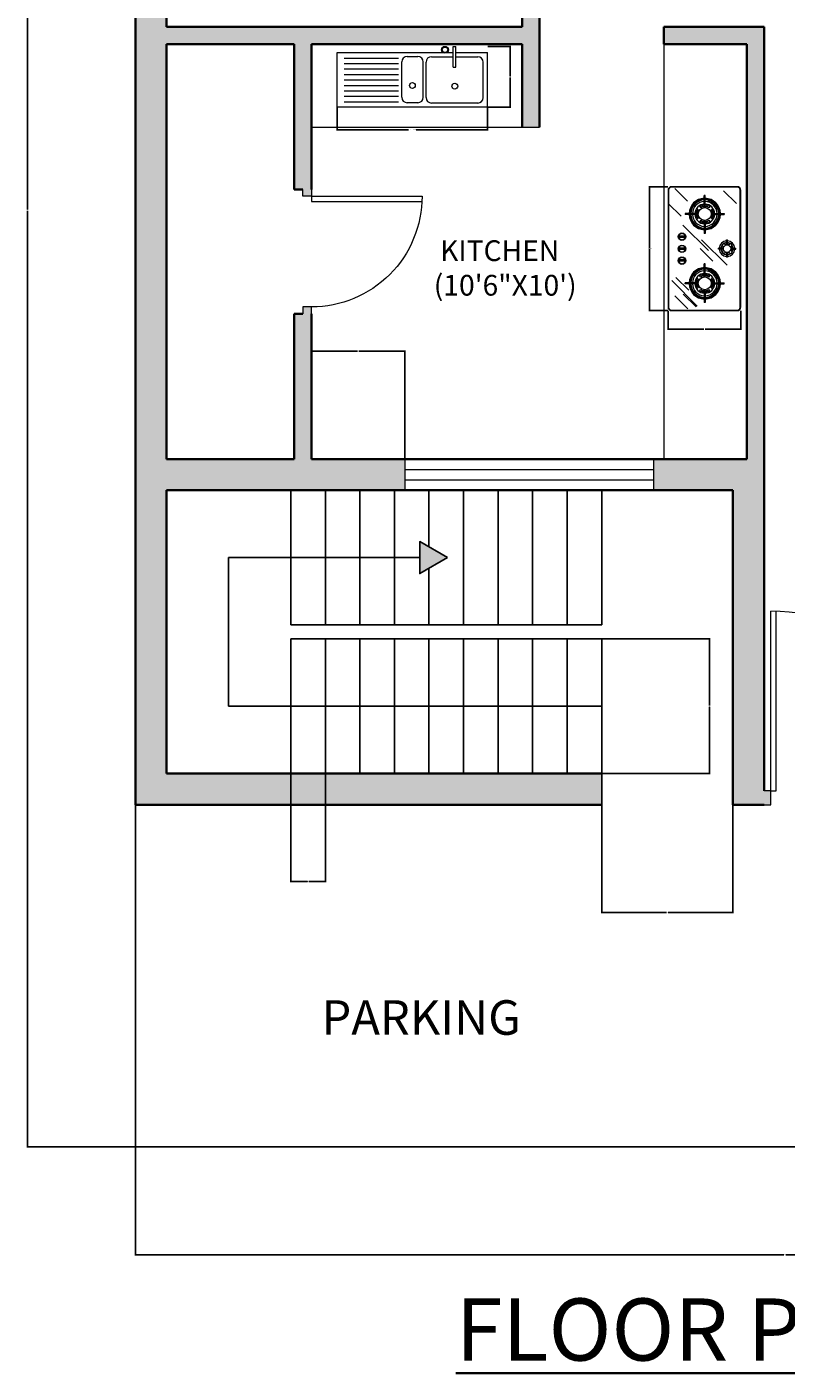
# Model space of a CAD drawing. Units: inches. Extents: x 2948 to 4025, y 2171 to 2966.
# Tile 1 of 6: x 2948 to 3168, y 2171 to 2560. Entities that reach past the tile are written whole.
import ezdxf

# ---------------------------------------------------------------- set-up
doc = ezdxf.new("R2010")
doc.units = ezdxf.units.IN
for name, color, linetype, lineweight in [('A-ANNO-DIMS', 2, 'Continuous', 18), ('A-ANNO-TEXT', 7, 'Continuous', 35), ('A-AREA-IDEN', 7, 'Continuous', 18), ('A-DOOR', 3, 'Continuous', 18), ('A-EQPM', 8, 'Continuous', 18), ('A-FLOR-CASE', 8, 'Continuous', 18), ('A-FLOR-FIXT', 9, 'Continuous', 18), ('A-FLOR-STRS', 7, 'Continuous', 25), ('A-GLAZ', 4, 'Continuous', 18), ('A-WALL', 7, 'Continuous', 35), ('A-WALL-PATT', 252, 'Continuous', 13)]:
    doc.layers.add(name, color=color, linetype=linetype, lineweight=lineweight)
doc.styles.get("Standard").update_dxf_attribs({"font": 'arial.ttf'})
doc.dimstyles.get("Standard").update_dxf_attribs({"dimtxt": 0.18, "dimasz": 0.18, "dimexe": 0.18, "dimexo": 0.0625, "dimgap": 0.09, "dimtad": 0, "dimtih": 1, "dimtoh": 1, "dimdec": 4, "dimzin": 0, "dimdsep": 46, "dimtxsty": 'Standard', "dimcen": 0.09, "dimadec": 0, "dimazin": 0, "dimtfac": 1, "dimtdec": 4, "dimtofl": 0, "dimtmove": 0, "dimatfit": 3, "dimfxl": 1, "dimtolj": 1, "dimtzin": 0, "dimarcsym": 0})

# ---------------------------------------------------------------- blocks, each defined once
blk = doc.blocks.new('A$C038F079D')
for p, q in [((23.9, 336.8), (101.3, 414.2)), ((377.5, 410.6), (372.5, 410.6)), ((320.9, 202.7), (475.7, 357.5)), ((427.1, 359.8), (427.1, 354.8)), ((587.4, 339.9), (582.4, 339.9)), ((377.5, 305.6), (372.5, 305.6)), ((374.2, 193.8), (451.6, 271.2)), ((53.2, 224.7), (53.2, 219.7)), ((130.3, 173.3), (141.1, 184.1)), ((137.3, 169), (142.6, 174.2)), ((232.1, 89.3), (386.9, 244.1)), ((284, 224.7), (284, 219.7)), ((466, 224.7), (466, 219.7)), ((567.6, 22.2), (722.4, 177)), ((650.5, 92.2), (727.9, 169.6)), ((701.8, 224.7), (701.8, 219.7)), ((10.1, 41), (87.5, 118.4)), ((549.9, 47.9), (627.2, 125.3)), ((587.4, 103.7), (582.4, 103.7)), ((661.4, 42), (738.7, 119.3)), ((100.9, 1.5), (178.3, 78.9))]:
    blk.add_line(p, q)
at = {"ltscale": 0.18}
for p, q in [((372.5, 384.7), (372.5, 410.6)), ((377.5, 384.7), (377.5, 410.6)), ((162.6, 339.9), (167.6, 339.9)), ((162.6, 267.1), (162.6, 339.9)), ((167.6, 267.1), (167.6, 339.9)), ((322.3, 354.8), (322.3, 359.8)), ((347.6, 359.8), (322.3, 359.8)), ((347.6, 354.8), (322.3, 354.8)), ((350.8, 370.2), (343.5, 377.5)), ((343.5, 337.2), (350.8, 344.5)), ((362.2, 381.5), (354.8, 388.8)), ((354.8, 325.8), (362.2, 333.1)), ((372.5, 329.9), (372.5, 305.6)), ((377.5, 329.9), (377.5, 305.6)), ((387.8, 381.5), (395.2, 388.8)), ((395.2, 325.8), (387.8, 333.1)), ((399.2, 370.2), (406.5, 377.5)), ((406.5, 337.2), (399.2, 344.5)), ((402.4, 359.8), (427.1, 359.8)), ((402.4, 354.8), (427.1, 354.8)), ((582.4, 267.1), (582.4, 339.9)), ((587.4, 267.1), (587.4, 339.9)), ((111.9, 250), (117.1, 244.7)), ((116.2, 257), (127, 246.2)), ((130.3, 271.1), (141.1, 260.3)), ((137.3, 275.4), (142.6, 270.2)), ((187.6, 270.2), (192.8, 275.4)), ((189, 260.3), (199.8, 271.1)), ((203.2, 246.2), (214, 257)), ((213.1, 244.7), (218.3, 250)), ((536.9, 244.7), (531.7, 250)), ((546.8, 246.2), (536, 257)), ((561, 260.3), (550.2, 271.1)), ((562.4, 270.2), (557.2, 275.4)), ((612.7, 275.4), (607.4, 270.2)), ((619.7, 271.1), (608.9, 260.3)), ((633.8, 257), (623, 246.2)), ((638.1, 250), (632.9, 244.7)), ((125.1, 224.7), (53.2, 224.7)), ((125.1, 219.7), (53.2, 219.7)), ((111.9, 194.5), (117.1, 199.7)), ((116.2, 187.5), (127, 198.3)), ((162.6, 177.3), (162.6, 103.7)), ((167.6, 177.3), (167.6, 103.7)), ((187.6, 174.2), (192.8, 169)), ((189, 184.1), (199.8, 173.3)), ((203.2, 198.3), (214, 187.5)), ((210, 224.7), (284, 224.7)), ((210, 219.7), (284, 219.7)), ((213.1, 199.7), (218.3, 194.5)), ((540, 224.7), (466, 224.7)), ((540, 219.7), (466, 219.7)), ((536.9, 199.7), (531.7, 194.5)), ((546.8, 198.3), (536, 187.5)), ((561, 184.1), (550.2, 173.3)), ((562.4, 174.2), (557.2, 169)), ((582.4, 177.3), (582.4, 103.7)), ((587.4, 177.3), (587.4, 103.7)), ((612.7, 169), (607.4, 174.2)), ((619.7, 173.3), (608.9, 184.1)), ((633.8, 187.5), (623, 198.3)), ((629.9, 224.7), (701.8, 224.7)), ((629.9, 219.7), (701.8, 219.7)), ((638.1, 194.5), (632.9, 199.7)), ((162.6, 103.7), (167.6, 103.7)), ((298.6, 99.8), (298.6, 69)), ((306.6, 99.8), (306.6, 69)), ((372, 99.8), (372, 69)), ((380, 99.8), (380, 69)), ((443.4, 99.8), (443.4, 69)), ((451.4, 99.8), (451.4, 69))]:
    blk.add_line(p, q, dxfattribs=at)
for points in [[(20, 0), (730, 0, 0.414214), (750, 20), (750, 420, 0.414214), (730, 440), (20, 440, 0.414214), (0, 420), (0, 20, 0.414214)], [(20, 3), (730, 3, 0.414214), (747, 20), (747, 420, 0.414214), (730, 437), (20, 437, 0.414214), (3, 420), (3, 20, 0.414214)]]:
    blk.add_lwpolyline(points, format="xyb", close=True)
for centre in [(345.9, 386.3), (89.1, 248.3), (94.7, 261.5), (509, 247.6), (514.6, 260.8)]:
    blk.add_circle(centre, 3.73)
for centre, radius in [((375, 357.3), 22.4), ((165.1, 222.2), 39), ((584.9, 222.2), 39), ((302.6, 84.4), 22.5), ((302.6, 84.4), 21.5), ((376, 84.4), 22.5), ((376, 84.4), 21.5), ((447.4, 84.4), 22.5), ((447.4, 84.4), 21.5)]:
    blk.add_circle(centre, radius, dxfattribs=at)
for centre, radius, start, end in [((375, 357.3), 47.4, 93.02552, 176.97448), ((375, 357.3), 47.4, 183.02552, 266.97448), ((375, 357.3), 37.4, 93.83631, 176.16369), ((375, 357.3), 37.4, 183.83631, 266.16369), ((346.8, 357.3), 2.62, 287.63178, 72.36822), ((375, 357.3), 27.4, 151.9979, 174.83836), ((375, 357.3), 27.4, 185.16164, 208.0021), ((375, 357.3), 27.4, 95.20298, 118.0021), ((375, 357.3), 27.4, 241.9979, 264.75693), ((375, 385), 2.52, 187.95053, 352.04947), ((375, 330), 2.5, 358.33173, 181.66827), ((375, 357.3), 47.4, 3.02552, 86.97448), ((375, 357.3), 37.4, 3.83631, 86.16369), ((375, 357.3), 27.4, 61.9979, 84.79702), ((375, 357.3), 47.4, 273.02552, 356.97448), ((375, 357.3), 37.4, 273.83631, 356.16369), ((375, 357.3), 27.4, 275.24307, 298.0021), ((375, 357.3), 27.4, 5.20601, 28.0021), ((375, 357.3), 27.4, 331.9979, 354.79399), ((402.7, 357.3), 2.52, 97.22361, 262.77639), ((165.1, 222.2), 95, 91.59175, 178.40825), ((165.1, 222.2), 90, 91.59175, 178.40825), ((165.1, 222.2), 85, 91.68541, 178.31459), ((165.1, 222.2), 75, 91.91021, 178.08979), ((165.1, 222.2), 60, 92.38802, 177.61198), ((165.1, 222.2), 53, 154.85389, 177.29637), ((165.1, 222.2), 45, 147.83959, 176.81526), ((165.1, 222.2), 45, 93.18474, 122.16041), ((165.1, 222.2), 53, 92.70363, 115.14611), ((165.1, 267.4), 2.52, 186.73537, 353.26463), ((165.1, 222.2), 90, 1.59175, 88.40825), ((165.1, 222.2), 85, 1.68541, 88.31459), ((165.1, 222.2), 75, 1.91021, 88.08979), ((165.1, 222.2), 60, 2.38802, 87.61198), ((165.1, 222.2), 53, 64.85389, 87.29637), ((165.1, 222.2), 45, 57.83959, 86.81526), ((165.1, 222.2), 95, 1.59175, 88.40825), ((165.1, 222.2), 45, 3.18474, 32.16041), ((165.1, 222.2), 53, 2.70363, 25.14611), ((584.9, 222.2), 95, 91.59175, 178.40825), ((584.9, 222.2), 90, 91.59175, 178.40825), ((584.9, 222.2), 85, 91.68541, 178.31459), ((584.9, 222.2), 75, 91.91021, 178.08979), ((584.9, 222.2), 60, 92.38802, 177.61198), ((584.9, 222.2), 53, 154.85389, 177.29637), ((584.9, 222.2), 45, 147.83959, 176.81526), ((584.9, 222.2), 45, 93.18474, 122.16041), ((584.9, 222.2), 53, 92.70363, 115.14611), ((584.9, 267.3), 2.51, 183.95793, 356.04207), ((584.9, 222.2), 90, 1.59175, 88.40825), ((584.9, 222.2), 85, 1.68541, 88.31459), ((584.9, 222.2), 75, 1.91021, 88.08979), ((584.9, 222.2), 60, 2.38802, 87.61198), ((584.9, 222.2), 53, 64.85389, 87.29637), ((584.9, 222.2), 45, 57.83959, 86.81526), ((584.9, 222.2), 95, 1.59175, 88.40825), ((584.9, 222.2), 45, 3.18474, 32.16041), ((584.9, 222.2), 53, 2.70363, 25.14611), ((165.1, 222.2), 95, 181.59175, 268.40825), ((165.1, 222.2), 90, 181.59175, 268.40825), ((165.1, 222.2), 85, 181.68541, 268.31459), ((165.1, 222.2), 75, 181.91021, 268.08979), ((165.1, 222.2), 60, 182.38802, 267.61198), ((165.1, 222.2), 53, 182.70363, 205.14611), ((119.3, 222.2), 2.64, 288.75105, 71.24895), ((165.1, 222.2), 45, 183.18474, 212.16041), ((165.1, 222.2), 45, 237.83959, 266.81526), ((165.1, 222.2), 53, 244.85389, 267.29637), ((165.1, 222.2), 75, 271.91021, 358.08979), ((165.1, 222.2), 60, 272.38802, 357.61198), ((165.1, 222.2), 85, 271.68541, 358.31459), ((165.1, 222.2), 90, 271.59175, 358.40825), ((165.1, 222.2), 45, 273.18474, 302.16041), ((165.1, 222.2), 53, 272.70363, 295.14611), ((165.1, 222.2), 95, 271.59175, 358.40825), ((165.1, 222.2), 45, 327.83959, 356.81526), ((210.9, 222.2), 2.67, 110.55069, 249.44931), ((165.1, 222.2), 53, 334.85389, 357.29637), ((584.9, 222.2), 95, 181.59175, 268.40825), ((584.9, 222.2), 90, 181.59175, 268.40825), ((584.9, 222.2), 85, 181.68541, 268.31459), ((584.9, 222.2), 75, 181.91021, 268.08979), ((584.9, 222.2), 60, 182.38802, 267.61198), ((584.9, 222.2), 53, 182.70363, 205.14611), ((539.2, 222.2), 2.63, 288.41197, 71.58803), ((584.9, 222.2), 45, 183.18474, 212.16041), ((584.9, 222.2), 45, 237.83959, 266.81526), ((584.9, 222.2), 53, 244.85389, 267.29637), ((584.9, 176.5), 2.63, 17.9418, 162.0582), ((584.9, 222.2), 90, 271.59175, 358.40825), ((584.9, 222.2), 85, 271.68541, 358.31459), ((584.9, 222.2), 75, 271.91021, 358.08979), ((584.9, 222.2), 60, 272.38802, 357.61198), ((584.9, 222.2), 45, 273.18474, 302.16041), ((584.9, 222.2), 53, 272.70363, 295.14611), ((584.9, 222.2), 95, 271.59175, 358.40825), ((584.9, 222.2), 45, 327.83959, 356.81526), ((630.5, 222.2), 2.58, 104.29448, 255.70552), ((584.9, 222.2), 53, 334.85389, 357.29637), ((302.6, 84.4), 18.5, 111.32369, 248.67631), ((296.6, 99.8), 2, 0, 111.32369), ((308.6, 99.8), 2, 68.67631, 180), ((302.6, 84.4), 18.5, 291.32369, 68.67631), ((376, 84.4), 18.5, 111.32369, 248.67631), ((370, 99.8), 2, 0, 111.32369), ((382, 99.8), 2, 68.67631, 180), ((376, 84.4), 18.5, 291.32369, 68.67631), ((447.4, 84.4), 18.5, 111.32369, 248.67631), ((441.4, 99.8), 2, 0, 111.32369), ((453.4, 99.8), 2, 68.67631, 180), ((447.4, 84.4), 18.5, 291.32369, 68.67631), ((296.6, 69), 2, 248.67631, 0), ((308.6, 69), 2, 180, 291.32369), ((370, 69), 2, 248.67631, 0), ((382, 69), 2, 180, 291.32369), ((441.4, 69), 2, 248.67631, 0), ((453.4, 69), 2, 180, 291.32369)]:
    blk.add_arc(centre, radius, start, end, dxfattribs=at)
blk.add_arc((165.1, 176.3), 2.69, 21.78852, 158.21148)
blk = doc.blocks.new('A$C5F013863')
at = {"ltscale": 1000}
for p, q in [((0, 400), (778.1, 400)), ((0, 0), (0, 400)), ((805.2, 400), (852.6, 400)), ((852.6, 293.9), (852.6, 446)), ((852.6, 446), (872.6, 446)), ((872.6, 293.9), (872.6, 446)), ((872.6, 400), (1104.6, 400)), ((1104.6, 0), (1104.6, 400)), ((50, 360), (450, 360)), ((50, 320), (450, 320)), ((473.8, 72.3), (473.8, 332.3)), ((513.8, 372.3), (592.2, 372.3)), ((632.2, 72.3), (632.2, 332.3)), ((652.6, 70), (652.6, 330)), ((692.6, 370), (852.6, 370)), ((872.6, 370), (1032.6, 370)), ((1072.6, 70), (1072.6, 330)), ((50, 280), (450, 280)), ((50, 240), (450, 240)), ((50, 200), (450, 200)), ((852.6, 293.9), (872.6, 293.9)), ((50, 160), (450, 160)), ((50, 120), (450, 120)), ((50, 80), (450, 80)), ((50, 40), (450, 40)), ((592.2, 32.3), (513.8, 32.3)), ((1032.6, 30), (692.6, 30)), ((1104.6, 0), (0, 0))]:
    blk.add_line(p, q, dxfattribs=at)
for centre, radius in [((791.7, 421), 25), ((791.7, 421), 20), ((552.4, 158.7), 21.4), ((863.5, 154.1), 21.4)]:
    blk.add_circle(centre, radius, dxfattribs=at)
for centre, start, end in [((513.8, 332.3), 90, 180), ((592.2, 332.3), 0, 90), ((692.6, 330), 90, 180), ((1032.6, 330), 0, 90), ((513.8, 72.3), 180, 270), ((592.2, 72.3), 270, 0), ((692.6, 70), 180, 270), ((1032.6, 70), 270, 0)]:
    blk.add_arc(centre, 40, start, end, dxfattribs=at)
blk = doc.blocks.new('DOOR-SWING-32IN')
for p, q in [((2, 34.5), (0, 34.5)), ((0, 32), (2, 32)), ((2, 32), (2, 34.5)), ((2, 32), (2, 0)), ((2, 32), (3.5, 32)), ((3.5, 32), (3.5, 0.04)), ((34, 32), (34, 34.5)), ((34, 34.5), (36, 34.5)), ((36, 32), (34, 32))]:
    blk.add_line(p, q)
blk.add_arc((2, 32), 32, 270, 0)
blk = doc.blocks.new('DOOR-ENTRY-52IN')
for p, q in [((2, 4), (2, 56)), ((3.5, 4), (3.5, 55.98)), ((2, 4), (0, 4)), ((2, 0), (2, 4)), ((2, 4), (3.5, 4)), ((54, 0), (54, 4)), ((54, 4), (56, 4)), ((0, 0), (2, 0)), ((56, 0), (54, 0))]:
    blk.add_line(p, q)
blk.add_arc((2, 4), 52, 0, 90)
blk = doc.blocks.new('WIN-72IN')
for p, q in [((0, 0), (0, 9)), ((72, 0), (72, 9)), ((72, 6), (0, 6)), ((72, 3), (0, 3))]:
    blk.add_line(p, q)
blk = doc.blocks.new('STAIR-RETURN-FLIGHT')
h = blk.add_hatch(color=256)
h.dxf.hatch_style = 1
h.paths.add_polyline_path([(63.35, 71.5), (55.35, 76.12), (55.35, 66.88)])
for p, q in [((18.02, 91), (18.02, 52)), ((28.02, 91), (28.02, 52)), ((38.02, 91), (38.02, 52)), ((48.02, 91), (48.02, 52)), ((58.02, 91), (58.02, 74.58)), ((68.02, 91), (68.02, 52)), ((78.02, 91), (78.02, 52)), ((88.02, 91), (88.02, 52)), ((98.02, 91), (98.02, 52)), ((108.02, 91), (108.02, 52)), ((0, 28.5), (0, 71.5)), ((55.35, 71.5), (0, 71.5)), ((58.02, 68.42), (58.02, 52)), ((18.02, 52), (108.02, 52)), ((18.02, 48), (108.02, 48)), ((18.02, 48), (18.02, 9)), ((28.02, 48), (28.02, 9)), ((38.02, 48), (38.02, 9)), ((48.02, 48), (48.02, 9)), ((58.02, 48), (58.02, 9)), ((68.02, 48), (68.02, 9)), ((78.02, 48), (78.02, 9)), ((88.02, 48), (88.02, 9)), ((98.02, 48), (98.02, 9)), ((108.02, 48), (108.02, 0)), ((108.02, 28.5), (0, 28.5))]:
    blk.add_line(p, q)
blk.add_lwpolyline([(63.35, 71.5), (55.35, 76.12), (55.35, 66.88)], close=True)
blk = doc.blocks.new('*D33')
at = {"layer": 'A-ANNO-DIMS', "color": 0, "lineweight": -2, "transparency": 16777216}
for p, q in [((3133.67, 2513.76), (3128.17, 2513.76)), ((3128.35, 2513.58), (3128.35, 2496.02)), ((3128.35, 2478.1), (3128.35, 2495.66)), ((3133.67, 2477.92), (3128.17, 2477.92))]:
    blk.add_line(p, q, dxfattribs=at)
at = {"layer": 'A-ANNO-DIMS', "color": 0, "transparency": 16777216}
for points in [[(3128.32, 2513.58), (3128.38, 2513.58), (3128.35, 2513.76)], [(3128.32, 2478.1), (3128.38, 2478.1), (3128.35, 2477.92)]]:
    blk.add_solid(points, dxfattribs=at)
at = {"layer": 'Defpoints', "color": 0, "transparency": 16777216}
for p in [(3133.73, 2513.76), (3128.35, 2477.92), (3133.73, 2477.92)]:
    blk.add_point(p, dxfattribs=at)
at = {"layer": 'A-ANNO-DIMS', "color": 0, "transparency": 16777216, "insert": (3128.35, 2495.84), "char_height": 0.18, "attachment_point": 5}
blk.add_mtext('\\A1;COOKTOP 36', dxfattribs=at)
blk = doc.blocks.new('*D34')
at = {"layer": 'A-ANNO-DIMS', "color": 0, "lineweight": -2, "transparency": 16777216}
for p, q in [((3133.73, 2477.86), (3133.73, 2472.37)), ((3154.75, 2477.86), (3154.75, 2472.37)), ((3133.91, 2472.55), (3144.04, 2472.55)), ((3154.57, 2472.55), (3144.45, 2472.55))]:
    blk.add_line(p, q, dxfattribs=at)
at = {"layer": 'A-ANNO-DIMS', "color": 0, "transparency": 16777216}
for points in [[(3133.91, 2472.58), (3133.91, 2472.52), (3133.73, 2472.55)], [(3154.57, 2472.58), (3154.57, 2472.52), (3154.75, 2472.55)]]:
    blk.add_solid(points, dxfattribs=at)
at = {"layer": 'Defpoints', "color": 0, "transparency": 16777216}
for p in [(3133.73, 2477.92), (3154.75, 2477.92), (3154.75, 2472.55)]:
    blk.add_point(p, dxfattribs=at)
at = {"layer": 'A-ANNO-DIMS', "color": 0, "transparency": 16777216, "insert": (3144.24, 2472.55), "char_height": 0.18, "attachment_point": 5}
blk.add_mtext('\\A1;21', dxfattribs=at)
blk = doc.blocks.new('*D35')
at = {"layer": 'A-ANNO-DIMS', "color": 0, "lineweight": -2, "transparency": 16777216}
for p, q in [((3037.95, 2536.72), (3037.95, 2530.07)), ((3081.48, 2536.72), (3081.48, 2530.07)), ((3038.13, 2530.25), (3058.58, 2530.25)), ((3081.3, 2530.25), (3060.84, 2530.25))]:
    blk.add_line(p, q, dxfattribs=at)
at = {"layer": 'A-ANNO-DIMS', "color": 0, "transparency": 16777216}
for points in [[(3038.13, 2530.28), (3038.13, 2530.22), (3037.95, 2530.25)], [(3081.3, 2530.28), (3081.3, 2530.22), (3081.48, 2530.25)]]:
    blk.add_solid(points, dxfattribs=at)
at = {"layer": 'Defpoints', "color": 0, "transparency": 16777216}
for p in [(3037.95, 2536.78), (3081.48, 2536.78), (3081.48, 2530.25)]:
    blk.add_point(p, dxfattribs=at)
at = {"layer": 'A-ANNO-DIMS', "color": 0, "transparency": 16777216, "insert": (3059.71, 2530.25), "char_height": 0.18, "attachment_point": 5}
blk.add_mtext('\\A1;KITCHEN SINK 44', dxfattribs=at)
blk = doc.blocks.new('*D36')
at = {"layer": 'A-ANNO-DIMS', "color": 0, "lineweight": -2, "transparency": 16777216}
for p, q in [((3081.54, 2554.36), (3088.19, 2554.36)), ((3088.01, 2554.18), (3088.01, 2545.75)), ((3088.01, 2536.96), (3088.01, 2545.39)), ((3081.54, 2536.78), (3088.19, 2536.78))]:
    blk.add_line(p, q, dxfattribs=at)
at = {"layer": 'A-ANNO-DIMS', "color": 0, "transparency": 16777216}
for points in [[(3087.98, 2554.18), (3088.04, 2554.18), (3088.01, 2554.36)], [(3087.98, 2536.96), (3088.04, 2536.96), (3088.01, 2536.78)]]:
    blk.add_solid(points, dxfattribs=at)
at = {"layer": 'Defpoints', "color": 0, "transparency": 16777216}
for p in [(3081.48, 2554.36), (3088.01, 2554.36), (3081.48, 2536.78)]:
    blk.add_point(p, dxfattribs=at)
at = {"layer": 'A-ANNO-DIMS', "color": 0, "transparency": 16777216, "insert": (3088.01, 2545.57), "char_height": 0.18, "attachment_point": 5}
blk.add_mtext('\\A1;18', dxfattribs=at)
blk = doc.blocks.new('*D37')
at = {"layer": 'A-ANNO-DIMS', "color": 0, "lineweight": -2, "transparency": 16777216}
for p, q in [((2979.51, 2334.92), (2979.51, 2204.61)), ((3355.51, 2235.92), (3355.51, 2204.61)), ((2979.69, 2204.79), (3167.22, 2204.79)), ((3355.33, 2204.79), (3167.8, 2204.79))]:
    blk.add_line(p, q, dxfattribs=at)
at = {"layer": 'A-ANNO-DIMS', "color": 0, "transparency": 16777216}
for points in [[(2979.69, 2204.82), (2979.69, 2204.76), (2979.51, 2204.79)], [(3355.33, 2204.82), (3355.33, 2204.76), (3355.51, 2204.79)]]:
    blk.add_solid(points, dxfattribs=at)
at = {"layer": 'Defpoints', "color": 0, "transparency": 16777216}
for p in [(2979.51, 2334.99), (3355.51, 2235.99), (3355.51, 2204.79)]:
    blk.add_point(p, dxfattribs=at)
at = {"layer": 'A-ANNO-DIMS', "color": 0, "transparency": 16777216, "insert": (3167.51, 2204.79), "char_height": 0.18, "attachment_point": 5}
blk.add_mtext('\\A1;376', dxfattribs=at)
blk = doc.blocks.new('*D38')
at = {"layer": 'A-ANNO-DIMS', "color": 0, "lineweight": -2, "transparency": 16777216}
for p, q in [((2979.45, 2777.99), (2948.13, 2777.99)), ((2948.31, 2777.81), (2948.31, 2507.17)), ((2948.31, 2236.17), (2948.31, 2506.8)), ((3217.45, 2235.99), (2948.13, 2235.99))]:
    blk.add_line(p, q, dxfattribs=at)
at = {"layer": 'A-ANNO-DIMS', "color": 0, "transparency": 16777216}
for points in [[(2948.28, 2777.81), (2948.34, 2777.81), (2948.31, 2777.99)], [(2948.28, 2236.17), (2948.34, 2236.17), (2948.31, 2235.99)]]:
    blk.add_solid(points, dxfattribs=at)
at = {"layer": 'Defpoints', "color": 0, "transparency": 16777216}
for p in [(2948.31, 2777.99), (2979.51, 2777.99), (3217.51, 2235.99)]:
    blk.add_point(p, dxfattribs=at)
at = {"layer": 'A-ANNO-DIMS', "color": 0, "transparency": 16777216, "insert": (2948.31, 2506.99), "char_height": 0.18, "attachment_point": 5}
blk.add_mtext('\\A1;542', dxfattribs=at)
blk = doc.blocks.new('*D43')
at = {"layer": 'A-ANNO-DIMS', "color": 0, "lineweight": -2, "transparency": 16777216}
for p, q in [((3030.51, 2435.05), (3030.51, 2466.37)), ((3030.69, 2466.19), (3043.79, 2466.19)), ((3057.33, 2466.19), (3044.23, 2466.19)), ((3057.51, 2435.05), (3057.51, 2466.37))]:
    blk.add_line(p, q, dxfattribs=at)
at = {"layer": 'A-ANNO-DIMS', "color": 0, "transparency": 16777216}
for points in [[(3030.69, 2466.22), (3030.69, 2466.16), (3030.51, 2466.19)], [(3057.33, 2466.22), (3057.33, 2466.16), (3057.51, 2466.19)]]:
    blk.add_solid(points, dxfattribs=at)
at = {"layer": 'Defpoints', "color": 0, "transparency": 16777216}
for p in [(3057.51, 2466.19), (3030.51, 2434.99), (3057.51, 2434.99)]:
    blk.add_point(p, dxfattribs=at)
at = {"layer": 'A-ANNO-DIMS', "color": 0, "transparency": 16777216, "insert": (3044.01, 2466.19), "char_height": 0.18, "attachment_point": 5}
blk.add_mtext('\\A1;27', dxfattribs=at)
blk = doc.blocks.new('*D46')
at = {"layer": 'A-ANNO-DIMS', "color": 0, "lineweight": -2, "transparency": 16777216}
for p, q in [((3114.51, 2334.92), (3114.51, 2303.61)), ((3152.51, 2334.92), (3152.51, 2303.61)), ((3114.69, 2303.79), (3133.29, 2303.79)), ((3152.33, 2303.79), (3133.73, 2303.79))]:
    blk.add_line(p, q, dxfattribs=at)
at = {"layer": 'A-ANNO-DIMS', "color": 0, "transparency": 16777216}
for points in [[(3114.69, 2303.82), (3114.69, 2303.76), (3114.51, 2303.79)], [(3152.33, 2303.82), (3152.33, 2303.76), (3152.51, 2303.79)]]:
    blk.add_solid(points, dxfattribs=at)
at = {"layer": 'Defpoints', "color": 0, "transparency": 16777216}
for p in [(3114.51, 2334.99), (3152.51, 2334.99), (3114.51, 2303.79)]:
    blk.add_point(p, dxfattribs=at)
at = {"layer": 'A-ANNO-DIMS', "color": 0, "transparency": 16777216, "insert": (3133.51, 2303.79), "char_height": 0.18, "attachment_point": 5}
blk.add_mtext('\\A1;38', dxfattribs=at)
blk = doc.blocks.new('*D47')
at = {"layer": 'A-ANNO-DIMS', "color": 0, "lineweight": -2, "transparency": 16777216}
for p, q in [((3024.51, 2343.92), (3024.51, 2312.61)), ((3034.51, 2343.92), (3034.51, 2312.61)), ((3024.69, 2312.79), (3029.3, 2312.79)), ((3034.33, 2312.79), (3029.72, 2312.79))]:
    blk.add_line(p, q, dxfattribs=at)
at = {"layer": 'A-ANNO-DIMS', "color": 0, "transparency": 16777216}
for points in [[(3024.69, 2312.82), (3024.69, 2312.76), (3024.51, 2312.79)], [(3034.33, 2312.82), (3034.33, 2312.76), (3034.51, 2312.79)]]:
    blk.add_solid(points, dxfattribs=at)
at = {"layer": 'Defpoints', "color": 0, "transparency": 16777216}
for p in [(3024.51, 2343.99), (3034.51, 2343.99), (3024.51, 2312.79)]:
    blk.add_point(p, dxfattribs=at)
at = {"layer": 'A-ANNO-DIMS', "color": 0, "transparency": 16777216, "insert": (3029.51, 2312.79), "char_height": 0.18, "attachment_point": 5}
blk.add_mtext('\\A1;10', dxfattribs=at)
blk = doc.blocks.new('*D48')
at = {"layer": 'A-ANNO-DIMS', "color": 0, "lineweight": -2, "transparency": 16777216}
for p, q in [((3114.58, 2382.99), (3145.89, 2382.99)), ((3145.71, 2382.81), (3145.71, 2363.67)), ((3145.71, 2344.17), (3145.71, 2363.3)), ((3114.58, 2343.99), (3145.89, 2343.99))]:
    blk.add_line(p, q, dxfattribs=at)
at = {"layer": 'A-ANNO-DIMS', "color": 0, "transparency": 16777216}
for points in [[(3145.68, 2382.81), (3145.74, 2382.81), (3145.71, 2382.99)], [(3145.68, 2344.17), (3145.74, 2344.17), (3145.71, 2343.99)]]:
    blk.add_solid(points, dxfattribs=at)
at = {"layer": 'Defpoints', "color": 0, "transparency": 16777216}
for p in [(3114.51, 2382.99), (3114.51, 2343.99), (3145.71, 2343.99)]:
    blk.add_point(p, dxfattribs=at)
at = {"layer": 'A-ANNO-DIMS', "color": 0, "transparency": 16777216, "insert": (3145.71, 2363.49), "char_height": 0.18, "attachment_point": 5}
blk.add_mtext('\\A1;39', dxfattribs=at)
blk = doc.blocks.new('*D67')
at = {"layer": 'A-ANNO-DIMS', "color": 0, "lineweight": -2, "transparency": 16777216}
for p, q in [((3222.34, 2397.82), (3200.41, 2375.88)), ((3222.52, 2397.82), (3222.34, 2397.82)), ((3163.42, 2338.99), (3163.6, 2338.99)), ((3163.51, 2338.9), (3163.51, 2339.08))]:
    blk.add_line(p, q, dxfattribs=at)
at = {"layer": 'A-ANNO-DIMS', "color": 0, "transparency": 16777216}
blk.add_solid([(3200.39, 2375.9), (3200.43, 2375.86), (3200.28, 2375.76)], dxfattribs=at)
at = {"layer": 'Defpoints', "color": 0, "transparency": 16777216}
for p in [(3200.28, 2375.76), (3163.51, 2338.99)]:
    blk.add_point(p, dxfattribs=at)
at = {"layer": 'A-ANNO-DIMS', "color": 0, "transparency": 16777216, "insert": (3222.83, 2397.82), "char_height": 0.18, "attachment_point": 5}
blk.add_mtext('\\A1;R52', dxfattribs=at)

msp = doc.modelspace()

# ---------------------------------------------------------------- hatches: boundary and pattern name
at = {"layer": 'A-WALL-PATT'}
h = msp.add_hatch(color=256, dxfattribs=at)
h.dxf.hatch_style = 1
h.paths.add_polyline_path([(3030.5136, 2476.9862), (3030.5136, 2478.9862), (3028.0136, 2478.9862), (3028.0136, 2476.9862), (3025.5136, 2476.9862), (3025.5136, 2434.9862), (2988.5136, 2434.9862), (2988.5136, 2554.9862), (3025.5136, 2554.9862), (3025.5136, 2512.9862), (3028.0136, 2512.9862), (3028.0136, 2510.9862), (3030.5136, 2510.9862), (3030.5136, 2512.9862), (3030.5136, 2554.9862), (3091.5136, 2554.9862), (3091.5136, 2530.9862), (3096.5136, 2530.9862), (3096.5136, 2622.4862), (3098.5136, 2622.4862), (3098.5136, 2624.9862), (3096.5136, 2624.9862), (3018.5136, 2624.9862), (3018.5136, 2622.4862), (3016.5136, 2622.4862), (3016.5136, 2619.9862), (3018.5136, 2619.9862), (3091.5136, 2619.9862), (3091.5136, 2559.9862), (2988.5136, 2559.9862), (2988.5136, 2577.9862), (2979.5136, 2577.9862), (2979.5136, 2334.9862), (3114.5136, 2334.9862), (3114.5136, 2343.9862), (2988.5136, 2343.9862), (2988.5136, 2425.9862), (3057.5136, 2425.9862), (3057.5136, 2434.9862), (3030.5136, 2434.9862)])
h = msp.add_hatch(color=256, dxfattribs=at)
h.dxf.hatch_style = 1
h.paths.add_polyline_path([(3161.5136, 2559.9862), (3132.5136, 2559.9862), (3132.5136, 2554.9862), (3156.5136, 2554.9862), (3156.5136, 2434.9862), (3129.5136, 2434.9862), (3129.5136, 2425.9862), (3152.5136, 2425.9862), (3152.5136, 2334.9862), (3161.5136, 2334.9862), (3163.5136, 2334.9862), (3163.5136, 2338.9862), (3161.5136, 2338.9862)])

# ---------------------------------------------------------------- linework, layer by layer
at = {"layer": 'A-FLOR-CASE'}
for p, q in [((3132.5136, 2559.9862), (3132.5136, 2434.9862)), ((3030.5136, 2530.9862), (3096.5136, 2530.9862))]:
    msp.add_line(p, q, dxfattribs=at)
at = {"layer": 'A-WALL'}
for p, q in [((2979.5136, 2777.9862), (2979.5136, 2334.9862)), ((3096.5136, 2622.4862), (3096.5136, 2530.9862)), ((2988.5136, 2619.9862), (2988.5136, 2559.9862)), ((3091.5136, 2619.9862), (3091.5136, 2559.9862)), ((2988.5136, 2559.9862), (3091.5136, 2559.9862)), ((3132.5136, 2559.9862), (3161.5136, 2559.9862)), ((3132.5136, 2559.9862), (3132.5136, 2554.9862)), ((3161.5136, 2559.9862), (3161.5136, 2338.9862)), ((2988.5136, 2554.9862), (3025.5136, 2554.9862)), ((2988.5136, 2554.9862), (2988.5136, 2434.9862)), ((3025.5136, 2554.9862), (3025.5136, 2512.9862)), ((3030.5136, 2554.9862), (3030.5136, 2512.9862)), ((3030.5136, 2554.9862), (3091.5136, 2554.9862)), ((3091.5136, 2554.9862), (3091.5136, 2530.9862)), ((3132.5136, 2554.9862), (3156.5136, 2554.9862)), ((3156.5136, 2554.9862), (3156.5136, 2434.9862)), ((3028.0136, 2512.9862), (3025.5136, 2512.9862)), ((3028.0136, 2476.9862), (3025.5136, 2476.9862)), ((3025.5136, 2476.9862), (3025.5136, 2434.9862)), ((3030.5136, 2476.9862), (3030.5136, 2434.9862)), ((2988.5136, 2434.9862), (3025.5136, 2434.9862)), ((3030.5136, 2434.9862), (3156.5136, 2434.9862)), ((2988.5136, 2425.9862), (3152.5136, 2425.9862)), ((2988.5136, 2425.9862), (2988.5136, 2343.9862)), ((3152.5136, 2425.9862), (3152.5136, 2334.9862)), ((2988.5136, 2343.9862), (3114.5136, 2343.9862)), ((2979.5136, 2334.9862), (3114.5136, 2334.9862)), ((3152.5136, 2334.9862), (3161.5136, 2334.9862))]:
    msp.add_line(p, q, dxfattribs=at)

# ---------------------------------------------------------------- block references
at = {"layer": 'A-DOOR', "extrusion": (0, 0, -1), "zscale": -1, "rotation": 269.9999999999993}
msp.add_blockref('DOOR-SWING-32IN', (-3062.5139, 2512.9859), dxfattribs=at)
at = {"layer": 'A-DOOR'}
msp.add_blockref('DOOR-ENTRY-52IN', (3161.514, 2334.986), dxfattribs=at)
at = {"layer": 'A-EQPM', "xscale": 0.0477834226823948, "yscale": 0.0477834226823948, "zscale": 0.0477834226823948, "rotation": 270}
msp.add_blockref('A$C038F079D', (3133.7299, 2513.7591), dxfattribs=at)
at = {"layer": 'A-FLOR-FIXT', "xscale": 0.0394088361911134, "yscale": 0.0394088361911134, "zscale": 0.0394088361911134}
msp.add_blockref('A$C5F013863', (3037.9471, 2536.7808), dxfattribs=at)
at = {"layer": 'A-FLOR-STRS'}
msp.add_blockref('STAIR-RETURN-FLIGHT', (3006.497, 2334.986), dxfattribs=at)
at = {"layer": 'A-GLAZ', "rotation": 180}
msp.add_blockref('WIN-72IN', (3129.5133, 2434.9864), dxfattribs=at)

# ---------------------------------------------------------------- texts
at = {"layer": 'A-ANNO-TEXT', "insert": (3072.2407, 2192.1642), "char_height": 18, "attachment_point": 1}
msp.add_mtext_dynamic_manual_height_columns('{\\LFLOOR PLAN}', width=162.804461, gutter_width=12.5, heights=[0], dxfattribs=at)
at = {"layer": 'A-AREA-IDEN', "attachment_point": 1}
for s, width, insert, char_height in [(' KITCHEN \\P(10\'6"X10\')', 59.378389, (3065.896, 2498.2583), 6), ('PARKING', 124.953177, (3033.3897, 2278.423), 10)]:
    msp.add_mtext_dynamic_manual_height_columns(s, width=width, gutter_width=12.5, heights=[0], dxfattribs=dict(at, insert=insert, char_height=char_height))

# ---------------------------------------------------------------- dimensions: what is measured, and where the dimension line sits
at = {"layer": 'A-ANNO-DIMS'}
for base, p1, p2, angle, picture, middle in [((2948.3136, 2777.9862), (3217.5136, 2235.9862), (2979.5136, 2777.9862), 90, '*D38', (2948.3136, 2506.9862)), ((3088.0082, 2554.3583), (3081.4785, 2536.7808), (3081.4785, 2554.3583), 90, '*D36', (3088.0082, 2545.5696)), ((3057.5136, 2466.1862), (3030.5136, 2434.9862), (3057.5136, 2434.9862), 0, '*D43', (3044.0136, 2466.1862)), ((3145.7136, 2343.9862), (3114.5136, 2382.9862), (3114.5136, 2343.9862), 270, '*D48', (3145.7136, 2363.4862)), ((3024.5136, 2312.7862), (3034.5136, 2343.9862), (3024.5136, 2343.9862), 180, '*D47', (3029.5136, 2312.7862)), ((3114.5136, 2303.7862), (3152.5136, 2334.9862), (3114.5136, 2334.9862), 180, '*D46', (3133.5136, 2303.7862))]:
    dim = msp.add_linear_dim(base=base, p1=p1, p2=p2, angle=angle, dimstyle='Standard', override={"dimdec": 0, "dimlfac": 1, "dimrnd": 0, "dimzin": 0, "dimdsep": 46, "dimlunit": 2}, dxfattribs=at)
    dim.commit()
    dim.dimension.update_dxf_attribs({"geometry": picture, "text_midpoint": middle})
dim = msp.add_linear_dim(base=(3081.4785, 2530.2511), p1=(3037.9471, 2536.7808), p2=(3081.4785, 2536.7808), text='KITCHEN SINK <>', dimstyle='Standard', override={"dimdec": 0, "dimlfac": 1, "dimrnd": 0, "dimzin": 0, "dimdsep": 46, "dimlunit": 2}, dxfattribs=at)
dim.commit()
dim.dimension.update_dxf_attribs({"geometry": '*D35', "text_midpoint": (3059.7128, 2530.2511)})
dim = msp.add_linear_dim(base=(3128.3543, 2477.9215), p1=(3133.7299, 2513.7591), p2=(3133.7299, 2477.9215), angle=270, text='COOKTOP <>', dimstyle='Standard', override={"dimdec": 0, "dimlfac": 1, "dimrnd": 0, "dimzin": 0, "dimdsep": 46, "dimlunit": 2}, dxfattribs=at)
dim.commit()
dim.dimension.update_dxf_attribs({"geometry": '*D33', "text_midpoint": (3128.3543, 2495.8403)})
for base, p1, p2, picture, middle in [((3154.7547, 2472.5459), (3133.7299, 2477.9215), (3154.7547, 2477.9215), '*D34', (3144.2423, 2472.5459)), ((3355.5136, 2204.7862), (2979.5136, 2334.9862), (3355.5136, 2235.9862), '*D37', (3167.5136, 2204.7862))]:
    dim = msp.add_linear_dim(base=base, p1=p1, p2=p2, dimstyle='Standard', override={"dimdec": 0, "dimlfac": 1, "dimrnd": 0, "dimzin": 0, "dimdsep": 46, "dimlunit": 2}, dxfattribs=at)
    dim.commit()
    dim.dimension.update_dxf_attribs({"geometry": picture, "text_midpoint": middle})
dim = msp.add_radius_dim(center=(3163.5136, 2338.9862), mpoint=(3200.283, 2375.756), dimstyle='Standard', override={"dimdec": 0, "dimlfac": 1, "dimrnd": 0, "dimzin": 0, "dimdsep": 46, "dimlunit": 2}, dxfattribs=at)
dim.commit()
dim.dimension.update_dxf_attribs({"geometry": '*D67', "text_midpoint": (3222.8287, 2397.8178), "dimtype": 164})

doc.saveas('drawing.dxf')
